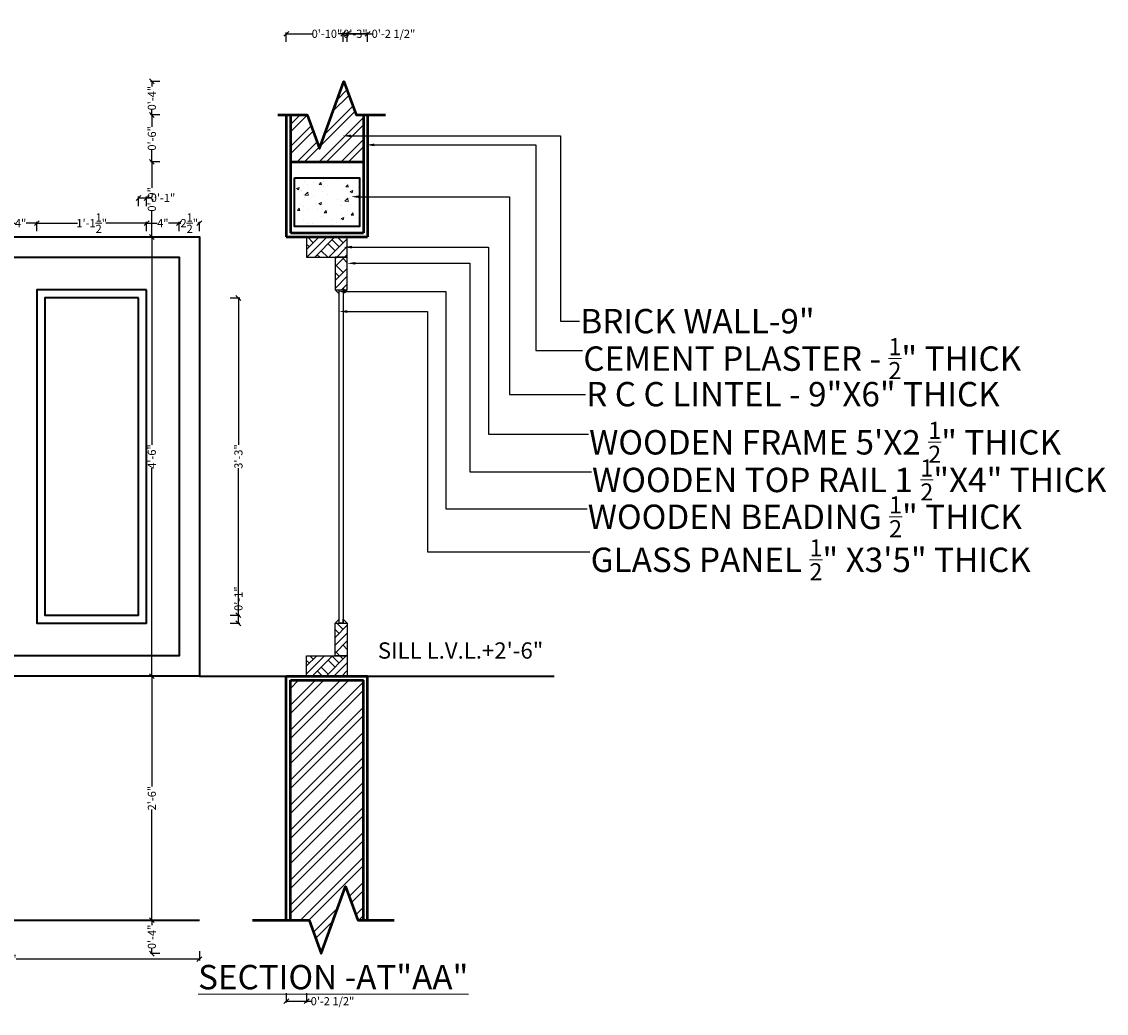
# Model space of a CAD drawing. Units: inches. Extents: x -54 to 163, y -154 to 48.
# Tile 3 of 3: x 30 to 163, y -74 to 48. Entities that reach past the tile are written whole.
import ezdxf
from ezdxf import colors
from ezdxf.entities.mleader import LeaderData, LeaderLine
from ezdxf.math import Vec2, Vec3

# ---------------------------------------------------------------- set-up
doc = ezdxf.new("R2010")
doc.units = ezdxf.units.IN
doc.header["$MEASUREMENT"] = 0
for name, color, linetype, lineweight in [('A-ANNO-DIMS', 2, 'Continuous', 18), ('A-ANNO-TEXT', 3, 'Continuous', 18), ('A-ELEV', 7, 'Continuous', 35), ('A-GLAZ', 4, 'Continuous', 25), ('A-GLAZ-PATT', 9, 'Continuous', 13), ('A-WALL', 7, 'Continuous', 50), ('A-WALL-PATT', 8, 'Continuous', 18), ('S-BEAM', 1, 'Continuous', 35)]:
    doc.layers.add(name, color=color, linetype=linetype, lineweight=lineweight)
doc.styles.get("Standard").update_dxf_attribs({"font": 'arial.ttf'})
doc.dimstyles.get("Standard").update_dxf_attribs({"dimtxt": 1, "dimasz": 0.6, "dimexe": 0.18, "dimexo": 0.0625, "dimgap": 0.09, "dimtad": 0, "dimdec": 1, "dimzin": 0, "dimdsep": 46, "dimlunit": 4, "dimtxsty": 'Standard', "dimblk": 'OBLIQUE', "dimcen": 0.09, "dimadec": 0, "dimazin": 0, "dimtfac": 1, "dimtdec": 1, "dimtofl": 0, "dimtmove": 0, "dimatfit": 3, "dimfxl": 1, "dimfxlon": 1, "dimtolj": 1, "dimtzin": 0, "dimarcsym": 0})

# ---------------------------------------------------------------- blocks, each defined once
blk = doc.blocks.new('_Oblique')
at = {"color": 0, "linetype": 'ByBlock', "lineweight": -2}
blk.add_line((-0.5, -0.5), (0.5, 0.5), dxfattribs=at)
blk = doc.blocks.new('*D6')
at = {"layer": 'A-ANNO-DIMS', "color": 0, "lineweight": -2, "transparency": 16777216}
for p, q in [((27.48, 22.51), (27.48, 23.69)), ((27.48, 23.51), (28.8, 23.51)), ((31.48, 23.51), (30.17, 23.51)), ((31.48, 22.51), (31.48, 23.69))]:
    blk.add_line(p, q, dxfattribs=at)
at = {"layer": 'Defpoints', "color": 0, "transparency": 16777216}
for p in [(31.48, 23.51), (27.48, 15.31), (31.48, 15.31)]:
    blk.add_point(p, dxfattribs=at)
at = {"layer": 'A-ANNO-DIMS', "color": 0, "lineweight": -2, "transparency": 16777216, "xscale": 0.6, "yscale": 0.6, "zscale": 0.6, "rotation": 180}
blk.add_blockref('_Oblique', (27.48, 23.51), dxfattribs=at)
at = {"layer": 'A-ANNO-DIMS', "color": 0, "lineweight": -2, "transparency": 16777216, "xscale": 0.6, "yscale": 0.6, "zscale": 0.6}
blk.add_blockref('_Oblique', (31.48, 23.51), dxfattribs=at)
at = {"layer": 'A-ANNO-DIMS', "color": 0, "transparency": 16777216, "insert": (29.48, 23.51), "char_height": 1, "attachment_point": 5}
blk.add_mtext('\\A1;4"', dxfattribs=at)
blk = doc.blocks.new('*D7')
at = {"layer": 'A-ANNO-DIMS', "color": 0, "lineweight": -2, "transparency": 16777216}
for p, q in [((31.48, 22.51), (31.48, 23.69)), ((31.48, 23.51), (36.49, 23.51)), ((44.98, 23.51), (39.97, 23.51)), ((44.98, 22.51), (44.98, 23.69))]:
    blk.add_line(p, q, dxfattribs=at)
at = {"layer": 'Defpoints', "color": 0, "transparency": 16777216}
for p in [(44.98, 23.51), (31.48, 15.31), (44.98, 15.31)]:
    blk.add_point(p, dxfattribs=at)
at = {"layer": 'A-ANNO-DIMS', "color": 0, "lineweight": -2, "transparency": 16777216, "xscale": 0.6, "yscale": 0.6, "zscale": 0.6, "rotation": 180}
blk.add_blockref('_Oblique', (31.48, 23.51), dxfattribs=at)
at = {"layer": 'A-ANNO-DIMS', "color": 0, "lineweight": -2, "transparency": 16777216, "xscale": 0.6, "yscale": 0.6, "zscale": 0.6}
blk.add_blockref('_Oblique', (44.98, 23.51), dxfattribs=at)
at = {"layer": 'A-ANNO-DIMS', "color": 0, "transparency": 16777216, "insert": (38.23, 23.51), "char_height": 1, "attachment_point": 5}
blk.add_mtext('\\A1;1\'-1{\\H1x;\\S1/2;}"', dxfattribs=at)
blk = doc.blocks.new('*D8')
at = {"layer": 'A-ANNO-DIMS', "color": 0, "lineweight": -2, "transparency": 16777216}
for p, q in [((44.98, 22.51), (44.98, 23.69)), ((44.98, 23.51), (46.3, 23.51)), ((48.98, 23.51), (47.67, 23.51)), ((48.98, 22.51), (48.98, 23.69))]:
    blk.add_line(p, q, dxfattribs=at)
at = {"layer": 'Defpoints', "color": 0, "transparency": 16777216}
for p in [(48.98, 23.51), (44.98, 15.31), (48.98, 15.31)]:
    blk.add_point(p, dxfattribs=at)
at = {"layer": 'A-ANNO-DIMS', "color": 0, "lineweight": -2, "transparency": 16777216, "xscale": 0.6, "yscale": 0.6, "zscale": 0.6, "rotation": 180}
blk.add_blockref('_Oblique', (44.98, 23.51), dxfattribs=at)
at = {"layer": 'A-ANNO-DIMS', "color": 0, "lineweight": -2, "transparency": 16777216, "xscale": 0.6, "yscale": 0.6, "zscale": 0.6}
blk.add_blockref('_Oblique', (48.98, 23.51), dxfattribs=at)
at = {"layer": 'A-ANNO-DIMS', "color": 0, "transparency": 16777216, "insert": (46.98, 23.51), "char_height": 1, "attachment_point": 5}
blk.add_mtext('\\A1;4"', dxfattribs=at)
blk = doc.blocks.new('*D9')
at = {"layer": 'A-ANNO-DIMS', "color": 0, "lineweight": -2, "transparency": 16777216}
for p, q in [((48.98, 22.51), (48.98, 23.69)), ((48.98, 23.51), (49.19, 23.51)), ((51.48, 23.51), (51.27, 23.51)), ((51.48, 22.51), (51.48, 23.69))]:
    blk.add_line(p, q, dxfattribs=at)
at = {"layer": 'Defpoints', "color": 0, "transparency": 16777216}
for p in [(51.48, 23.51), (48.98, 19.31), (51.48, 19.31)]:
    blk.add_point(p, dxfattribs=at)
at = {"layer": 'A-ANNO-DIMS', "color": 0, "lineweight": -2, "transparency": 16777216, "xscale": 0.6, "yscale": 0.6, "zscale": 0.6, "rotation": 180}
blk.add_blockref('_Oblique', (48.98, 23.51), dxfattribs=at)
at = {"layer": 'A-ANNO-DIMS', "color": 0, "lineweight": -2, "transparency": 16777216, "xscale": 0.6, "yscale": 0.6, "zscale": 0.6}
blk.add_blockref('_Oblique', (51.48, 23.51), dxfattribs=at)
at = {"layer": 'A-ANNO-DIMS', "color": 0, "transparency": 16777216, "insert": (50.23, 23.51), "char_height": 1, "attachment_point": 5}
blk.add_mtext('\\A1;2{\\H1x;\\S1/2;}"', dxfattribs=at)
blk = doc.blocks.new('*D18')
at = {"layer": 'A-ANNO-DIMS', "color": 0, "lineweight": -2, "transparency": 16777216}
for p, q in [((3.48, -65.99), (3.48, -67.17)), ((51.48, -65.99), (51.48, -67.17)), ((3.48, -66.99), (26.04, -66.99)), ((51.48, -66.99), (28.92, -66.99))]:
    blk.add_line(p, q, dxfattribs=at)
at = {"layer": 'Defpoints', "color": 0, "transparency": 16777216}
for p in [(3.48, -62.19), (51.48, -62.19), (51.48, -66.99)]:
    blk.add_point(p, dxfattribs=at)
at = {"layer": 'A-ANNO-DIMS', "color": 0, "lineweight": -2, "transparency": 16777216, "xscale": 0.6, "yscale": 0.6, "zscale": 0.6, "rotation": 180}
blk.add_blockref('_Oblique', (3.48, -66.99), dxfattribs=at)
at = {"layer": 'A-ANNO-DIMS', "color": 0, "lineweight": -2, "transparency": 16777216, "xscale": 0.6, "yscale": 0.6, "zscale": 0.6}
blk.add_blockref('_Oblique', (51.48, -66.99), dxfattribs=at)
at = {"layer": 'A-ANNO-DIMS', "color": 0, "transparency": 16777216, "insert": (27.48, -66.99), "char_height": 1, "attachment_point": 5}
blk.add_mtext('\\A1;4\'-0"', dxfattribs=at)
blk = doc.blocks.new('*D20')
at = {"layer": 'A-ANNO-DIMS', "color": 0, "lineweight": -2, "transparency": 16777216}
for p, q in [((55.28, 14.31), (56.46, 14.31)), ((56.28, 14.31), (56.28, -3.77)), ((56.28, -24.69), (56.28, -6.6)), ((55.28, -24.69), (56.46, -24.69))]:
    blk.add_line(p, q, dxfattribs=at)
at = {"layer": 'Defpoints', "color": 0, "transparency": 16777216}
for p in [(10.98, 14.31), (10.98, -24.69), (56.28, -24.69)]:
    blk.add_point(p, dxfattribs=at)
at = {"layer": 'A-ANNO-DIMS', "color": 0, "lineweight": -2, "transparency": 16777216, "xscale": 0.6, "yscale": 0.6, "zscale": 0.6}
for p, rotation in [((56.28, 14.31), 90), ((56.28, -24.69), 270)]:
    blk.add_blockref('_Oblique', p, dxfattribs=dict(at, rotation=rotation))
at = {"layer": 'A-ANNO-DIMS', "color": 0, "transparency": 16777216, "insert": (56.28, -5.19), "char_height": 1, "attachment_point": 5, "rotation": 90}
blk.add_mtext('\\A1;3\'-3"', dxfattribs=at)
blk = doc.blocks.new('*D21')
at = {"layer": 'A-ANNO-DIMS', "color": 0, "lineweight": -2, "transparency": 16777216}
for p, q in [((43.98, 25.61), (43.98, 26.79)), ((44.98, 25.61), (44.98, 26.79)), ((43.98, 26.61), (44.98, 26.61)), ((44.98, 26.61), (45.58, 26.61))]:
    blk.add_line(p, q, dxfattribs=at)
at = {"layer": 'Defpoints', "color": 0, "transparency": 16777216}
for p in [(44.98, 26.61), (44.98, 15.31), (43.98, 14.31)]:
    blk.add_point(p, dxfattribs=at)
at = {"layer": 'A-ANNO-DIMS', "color": 0, "lineweight": -2, "transparency": 16777216, "xscale": 0.6, "yscale": 0.6, "zscale": 0.6, "rotation": 180}
blk.add_blockref('_Oblique', (43.98, 26.61), dxfattribs=at)
at = {"layer": 'A-ANNO-DIMS', "color": 0, "lineweight": -2, "transparency": 16777216, "xscale": 0.6, "yscale": 0.6, "zscale": 0.6}
blk.add_blockref('_Oblique', (44.98, 26.61), dxfattribs=at)
at = {"layer": 'A-ANNO-DIMS', "color": 0, "transparency": 16777216, "insert": (47, 26.61), "char_height": 1, "attachment_point": 5}
blk.add_mtext('\\A1;0\'-1"', dxfattribs=at)
blk = doc.blocks.new('*D22')
at = {"layer": 'A-ANNO-DIMS', "color": 0, "lineweight": -2, "transparency": 16777216}
for p, q in [((55.28, -24.69), (56.46, -24.69)), ((56.28, -24.69), (56.28, -24.09)), ((56.28, -25.69), (56.28, -24.69)), ((55.28, -25.69), (56.46, -25.69))]:
    blk.add_line(p, q, dxfattribs=at)
at = {"layer": 'Defpoints', "color": 0, "transparency": 16777216}
for p in [(43.98, -24.69), (56.28, -24.69), (44.98, -25.69)]:
    blk.add_point(p, dxfattribs=at)
at = {"layer": 'A-ANNO-DIMS', "color": 0, "lineweight": -2, "transparency": 16777216, "xscale": 0.6, "yscale": 0.6, "zscale": 0.6}
for p, rotation in [((56.28, -24.69), 90), ((56.28, -25.69), 270)]:
    blk.add_blockref('_Oblique', p, dxfattribs=dict(at, rotation=rotation))
at = {"layer": 'A-ANNO-DIMS', "color": 0, "transparency": 16777216, "insert": (56.28, -22.67), "char_height": 1, "attachment_point": 5, "rotation": 90}
blk.add_mtext('\\A1;0\'-1"', dxfattribs=at)
blk = doc.blocks.new('*D23')
at = {"layer": 'A-ANNO-DIMS', "color": 0, "lineweight": -2, "transparency": 16777216}
for p, q in [((62.17, 45.79), (62.17, 46.97)), ((62.17, 46.79), (65.36, 46.79)), ((72.17, 46.79), (68.97, 46.79)), ((72.17, 45.79), (72.17, 46.97))]:
    blk.add_line(p, q, dxfattribs=at)
at = {"layer": 'Defpoints', "color": 0, "transparency": 16777216}
for p in [(72.17, 46.79), (62.17, 36.81), (72.17, 36.81)]:
    blk.add_point(p, dxfattribs=at)
at = {"layer": 'A-ANNO-DIMS', "color": 0, "lineweight": -2, "transparency": 16777216, "xscale": 0.6, "yscale": 0.6, "zscale": 0.6, "rotation": 180}
blk.add_blockref('_Oblique', (62.17, 46.79), dxfattribs=at)
at = {"layer": 'A-ANNO-DIMS', "color": 0, "lineweight": -2, "transparency": 16777216, "xscale": 0.6, "yscale": 0.6, "zscale": 0.6}
blk.add_blockref('_Oblique', (72.17, 46.79), dxfattribs=at)
at = {"layer": 'A-ANNO-DIMS', "color": 0, "transparency": 16777216, "insert": (67.17, 46.79), "char_height": 1, "attachment_point": 5}
blk.add_mtext('\\A1;0\'-10"', dxfattribs=at)
blk = doc.blocks.new('*D24')
at = {"layer": 'A-ANNO-DIMS', "color": 0, "lineweight": -2, "transparency": 16777216}
for p, q in [((46.63, 40.94), (45.45, 40.94)), ((45.63, 40.94), (45.63, 40.29)), ((45.63, 36.81), (45.63, 37.46)), ((46.63, 36.81), (45.45, 36.81))]:
    blk.add_line(p, q, dxfattribs=at)
at = {"layer": 'Defpoints', "color": 0, "transparency": 16777216}
for p in [(69.25, 40.94), (45.63, 36.81), (62.17, 36.81)]:
    blk.add_point(p, dxfattribs=at)
at = {"layer": 'A-ANNO-DIMS', "color": 0, "lineweight": -2, "transparency": 16777216, "xscale": 0.6, "yscale": 0.6, "zscale": 0.6}
for p, rotation in [((45.63, 40.94), 90), ((45.63, 36.81), 270)]:
    blk.add_blockref('_Oblique', p, dxfattribs=dict(at, rotation=rotation))
at = {"layer": 'A-ANNO-DIMS', "color": 0, "transparency": 16777216, "insert": (45.63, 38.88), "char_height": 1, "attachment_point": 5, "rotation": 90}
blk.add_mtext('\\A1;0\'-4"', dxfattribs=at)
blk = doc.blocks.new('*D25')
at = {"layer": 'A-ANNO-DIMS', "color": 0, "lineweight": -2, "transparency": 16777216}
for p, q in [((46.63, 36.81), (45.45, 36.81)), ((45.63, 36.81), (45.63, 35.35)), ((45.63, 31.05), (45.63, 32.51)), ((46.63, 31.05), (45.45, 31.05))]:
    blk.add_line(p, q, dxfattribs=at)
at = {"layer": 'Defpoints', "color": 0, "transparency": 16777216}
for p in [(62.17, 36.81), (45.63, 31.05), (62.67, 31.05)]:
    blk.add_point(p, dxfattribs=at)
at = {"layer": 'A-ANNO-DIMS', "color": 0, "lineweight": -2, "transparency": 16777216, "xscale": 0.6, "yscale": 0.6, "zscale": 0.6}
for p, rotation in [((45.63, 36.81), 90), ((45.63, 31.05), 270)]:
    blk.add_blockref('_Oblique', p, dxfattribs=dict(at, rotation=rotation))
at = {"layer": 'A-ANNO-DIMS', "color": 0, "transparency": 16777216, "insert": (45.63, 33.93), "char_height": 1, "attachment_point": 5, "rotation": 90}
blk.add_mtext('\\A1;0\'-6"', dxfattribs=at)
blk = doc.blocks.new('*D26')
at = {"layer": 'A-ANNO-DIMS', "color": 0, "lineweight": -2, "transparency": 16777216}
for p, q in [((46.63, 31.05), (45.45, 31.05)), ((45.63, 31.05), (45.63, 27.85)), ((45.63, 21.81), (45.63, 25.01)), ((46.63, 21.81), (45.45, 21.81))]:
    blk.add_line(p, q, dxfattribs=at)
at = {"layer": 'Defpoints', "color": 0, "transparency": 16777216}
for p in [(62.67, 31.05), (45.63, 21.81), (62.17, 21.81)]:
    blk.add_point(p, dxfattribs=at)
at = {"layer": 'A-ANNO-DIMS', "color": 0, "lineweight": -2, "transparency": 16777216, "xscale": 0.6, "yscale": 0.6, "zscale": 0.6}
for p, rotation in [((45.63, 31.05), 90), ((45.63, 21.81), 270)]:
    blk.add_blockref('_Oblique', p, dxfattribs=dict(at, rotation=rotation))
at = {"layer": 'A-ANNO-DIMS', "color": 0, "transparency": 16777216, "insert": (45.63, 26.43), "char_height": 1, "attachment_point": 5, "rotation": 90}
blk.add_mtext('\\A1;0\'-9"', dxfattribs=at)
blk = doc.blocks.new('*D27')
at = {"layer": 'A-ANNO-DIMS', "color": 0, "lineweight": -2, "transparency": 16777216}
for p, q in [((46.63, 21.81), (45.45, 21.81)), ((45.63, 21.81), (45.63, -3.75)), ((45.63, -32.19), (45.63, -6.62)), ((46.63, -32.19), (45.45, -32.19))]:
    blk.add_line(p, q, dxfattribs=at)
at = {"layer": 'Defpoints', "color": 0, "transparency": 16777216}
for p in [(62.17, 21.81), (45.63, -32.19), (62.17, -32.19)]:
    blk.add_point(p, dxfattribs=at)
at = {"layer": 'A-ANNO-DIMS', "color": 0, "lineweight": -2, "transparency": 16777216, "xscale": 0.6, "yscale": 0.6, "zscale": 0.6}
for p, rotation in [((45.63, 21.81), 90), ((45.63, -32.19), 270)]:
    blk.add_blockref('_Oblique', p, dxfattribs=dict(at, rotation=rotation))
at = {"layer": 'A-ANNO-DIMS', "color": 0, "transparency": 16777216, "insert": (45.63, -5.19), "char_height": 1, "attachment_point": 5, "rotation": 90}
blk.add_mtext('\\A1;4\'-6"', dxfattribs=at)
blk = doc.blocks.new('*D28')
at = {"layer": 'A-ANNO-DIMS', "color": 0, "lineweight": -2, "transparency": 16777216}
for p, q in [((46.63, -32.19), (45.45, -32.19)), ((45.63, -32.19), (45.63, -45.76)), ((45.63, -62.19), (45.63, -48.61)), ((46.63, -62.19), (45.45, -62.19))]:
    blk.add_line(p, q, dxfattribs=at)
at = {"layer": 'Defpoints', "color": 0, "transparency": 16777216}
for p in [(62.17, -32.19), (45.63, -62.19), (62.17, -62.19)]:
    blk.add_point(p, dxfattribs=at)
at = {"layer": 'A-ANNO-DIMS', "color": 0, "lineweight": -2, "transparency": 16777216, "xscale": 0.6, "yscale": 0.6, "zscale": 0.6}
for p, rotation in [((45.63, -32.19), 90), ((45.63, -62.19), 270)]:
    blk.add_blockref('_Oblique', p, dxfattribs=dict(at, rotation=rotation))
at = {"layer": 'A-ANNO-DIMS', "color": 0, "transparency": 16777216, "insert": (45.63, -47.19), "char_height": 1, "attachment_point": 5, "rotation": 90}
blk.add_mtext('\\A1;2\'-6"', dxfattribs=at)
blk = doc.blocks.new('*D29')
at = {"layer": 'A-ANNO-DIMS', "color": 0, "lineweight": -2, "transparency": 16777216}
for p, q in [((46.63, -62.19), (45.45, -62.19)), ((45.63, -62.19), (45.63, -62.83)), ((46.63, -66.31), (45.45, -66.31)), ((45.63, -66.31), (45.63, -65.67))]:
    blk.add_line(p, q, dxfattribs=at)
at = {"layer": 'Defpoints', "color": 0, "transparency": 16777216}
for p in [(62.17, -62.19), (45.63, -66.31), (66.46, -66.31)]:
    blk.add_point(p, dxfattribs=at)
at = {"layer": 'A-ANNO-DIMS', "color": 0, "lineweight": -2, "transparency": 16777216, "xscale": 0.6, "yscale": 0.6, "zscale": 0.6}
for p, rotation in [((45.63, -62.19), 90), ((45.63, -66.31), 270)]:
    blk.add_blockref('_Oblique', p, dxfattribs=dict(at, rotation=rotation))
at = {"layer": 'A-ANNO-DIMS', "color": 0, "transparency": 16777216, "insert": (45.63, -64.25), "char_height": 1, "attachment_point": 5, "rotation": 90}
blk.add_mtext('\\A1;0\'-4"', dxfattribs=at)
blk = doc.blocks.new('*D30')
at = {"layer": 'A-ANNO-DIMS', "color": 0, "lineweight": -2, "transparency": 16777216}
for p, q in [((69.67, 45.79), (69.67, 46.97)), ((69.67, 46.79), (72.17, 46.79)), ((72.17, 45.79), (72.17, 46.97)), ((72.17, 46.79), (72.77, 46.79))]:
    blk.add_line(p, q, dxfattribs=at)
at = {"layer": 'Defpoints', "color": 0, "transparency": 16777216}
for p in [(72.17, 46.79), (69.67, -32.19), (72.17, -32.19)]:
    blk.add_point(p, dxfattribs=at)
at = {"layer": 'A-ANNO-DIMS', "color": 0, "lineweight": -2, "transparency": 16777216, "xscale": 0.6, "yscale": 0.6, "zscale": 0.6, "rotation": 180}
blk.add_blockref('_Oblique', (69.67, 46.79), dxfattribs=at)
at = {"layer": 'A-ANNO-DIMS', "color": 0, "lineweight": -2, "transparency": 16777216, "xscale": 0.6, "yscale": 0.6, "zscale": 0.6}
blk.add_blockref('_Oblique', (72.17, 46.79), dxfattribs=at)
at = {"layer": 'A-ANNO-DIMS', "color": 0, "transparency": 16777216, "insert": (75.35, 46.79), "char_height": 1, "attachment_point": 5}
blk.add_mtext('\\A1;0\'-2 1/2"', dxfattribs=at)
blk = doc.blocks.new('*D31')
at = {"layer": 'A-ANNO-DIMS', "color": 0, "lineweight": -2, "transparency": 16777216}
for p, q in [((69.165189, 46.786945), (68.565189, 46.786945)), ((69.165189, 45.786945), (69.165189, 46.966945)), ((72.165189, 45.786945), (72.165189, 46.966945)), ((72.165189, 46.786945), (72.765189, 46.786945))]:
    blk.add_line(p, q, dxfattribs=at)
at = {"layer": 'Defpoints', "color": 0, "transparency": 16777216}
for p in [(72.165189, 46.786945), (69.165189, -25.685371), (72.165189, -32.185371)]:
    blk.add_point(p, dxfattribs=at)
at = {"layer": 'A-ANNO-DIMS', "color": 0, "lineweight": -2, "transparency": 16777216, "xscale": 0.6, "yscale": 0.6, "zscale": 0.6}
blk.add_blockref('_Oblique', (69.165189, 46.786945), dxfattribs=at)
at = {"layer": 'A-ANNO-DIMS', "color": 0, "lineweight": -2, "transparency": 16777216, "xscale": 0.6, "yscale": 0.6, "zscale": 0.6, "rotation": 180}
blk.add_blockref('_Oblique', (72.165189, 46.786945), dxfattribs=at)
at = {"layer": 'A-ANNO-DIMS', "color": 0, "transparency": 16777216, "insert": (70.665189, 46.786945), "char_height": 1, "attachment_point": 5}
blk.add_mtext('\\A1;0\'-3"', dxfattribs=at)
blk = doc.blocks.new('*D32')
at = {"layer": 'A-ANNO-DIMS', "color": 0, "lineweight": -2, "transparency": 16777216}
for p, q in [((62.17, -71.16), (62.17, -72.34)), ((64.67, -71.16), (64.67, -72.34)), ((62.17, -72.16), (64.67, -72.16)), ((64.67, -72.16), (65.27, -72.16))]:
    blk.add_line(p, q, dxfattribs=at)
at = {"layer": 'Defpoints', "color": 0, "transparency": 16777216}
for p in [(62.17, 21.81), (64.67, 21.81), (64.67, -72.16)]:
    blk.add_point(p, dxfattribs=at)
at = {"layer": 'A-ANNO-DIMS', "color": 0, "lineweight": -2, "transparency": 16777216, "xscale": 0.6, "yscale": 0.6, "zscale": 0.6, "rotation": 180}
blk.add_blockref('_Oblique', (62.17, -72.16), dxfattribs=at)
at = {"layer": 'A-ANNO-DIMS', "color": 0, "lineweight": -2, "transparency": 16777216, "xscale": 0.6, "yscale": 0.6, "zscale": 0.6}
blk.add_blockref('_Oblique', (64.67, -72.16), dxfattribs=at)
at = {"layer": 'A-ANNO-DIMS', "color": 0, "transparency": 16777216, "insert": (67.85, -72.16), "char_height": 1, "attachment_point": 5}
blk.add_mtext('\\A1;0\'-2 1/2"', dxfattribs=at)

msp = doc.modelspace()

# ---------------------------------------------------------------- hatches: boundary and pattern name
at = {"layer": 'A-GLAZ-PATT'}
h = msp.add_hatch(dxfattribs=at)
h.set_pattern_fill('º»ÊµÍÁÈÀ', color=256, scale=0.46)
h.set_pattern_definition([(45, (0.5428, 0), (-1.82801, 1.82801), []), (45, (1.5088, 0), (-1.82801, 1.82801), []), (45, (2.4748, 0), (-1.82801, 1.82801), []), (135, (0.5428, 0), (-1.82801, -1.82801), [1.219, -1.3662]), (135, (1.0258, 0.483), (-1.82801, -1.82801), [1.219, -1.3662]), (135, (1.5088, 0.966), (-1.82801, -1.82801), [1.219, -1.3662])])
h.paths.add_polyline_path([(69.67, 21.81), (64.67, 21.81), (64.67, 19.31), (69.67, 19.31)])
h.paths.add_polyline_path([(68.17, 15.31), (69.67, 15.31), (69.67, 19.31), (68.17, 19.31)])
h.paths.add_polyline_path([(68.17, -29.69), (64.67, -29.69), (64.67, -32.19), (69.67, -32.19), (69.67, -29.69)])
h.paths.add_polyline_path([(69.67, -25.69), (68.17, -25.69), (68.17, -29.69), (69.67, -29.69)])
at = {"layer": 'A-WALL-PATT'}
h = msp.add_hatch(dxfattribs=at)
h.set_pattern_fill('ANSI32', color=256, scale=5.1)
h.paths.add_polyline_path([(71.67, 36.81), (70.75, 36.81), (69.25, 40.94), (66.25, 32.69), (64.75, 36.81), (62.67, 36.81), (62.67, 31.05), (71.67, 31.05)])
h = msp.add_hatch(dxfattribs=at)
h.set_pattern_fill('AR-CONC', color=256, scale=0.46)
h.paths.add_polyline_path([(71.18, 29.08), (63.18, 29.08), (63.18, 23.08), (71.18, 23.08)])
h = msp.add_hatch(dxfattribs=at)
h.set_pattern_fill('ANSI32', color=256, scale=5.8)
h.paths.add_polyline_path([(71.67, -32.69), (62.67, -32.69), (62.67, -62.19), (64.96, -62.19), (66.46, -66.31), (69.46, -58.06), (70.96, -62.19), (71.67, -62.19)])

# ---------------------------------------------------------------- linework, layer by layer
at = {"layer": 'A-ELEV'}
for p, q in [((51.48, -32.19), (95.13, -32.19)), ((-20.18, -62.19), (51.48, -62.19))]:
    msp.add_line(p, q, dxfattribs=at)
msp.add_lwpolyline([(3.48, 21.81), (51.48, 21.81), (51.48, 19.31), (51.48, -29.69), (51.48, -32.19), (3.48, -32.19), (3.48, 21.81)], dxfattribs=at)
for points in [[(5.98, 19.31), (48.98, 19.31), (48.98, -29.69), (5.98, -29.69)], [(44.98, 15.31), (31.48, 15.31), (31.48, -25.69), (44.98, -25.69)], [(43.98, 14.31), (32.48, 14.31), (32.48, -24.69), (43.98, -24.69)]]:
    msp.add_lwpolyline(points, close=True, dxfattribs=at)
at = {"layer": 'A-GLAZ'}
for p, q in [((68.67, 14.81), (68.17, 15.31)), ((69.17, 14.81), (69.67, 15.31)), ((68.67, -25.19), (68.17, -25.69)), ((69.17, -25.69), (69.17, -25.19)), ((69.17, -25.19), (69.67, -25.69))]:
    msp.add_line(p, q, dxfattribs=at)
for points in [[(64.67, 19.31), (69.67, 19.31), (69.67, 21.81), (64.67, 21.81)], [(68.17, 15.31), (69.67, 15.31), (69.67, 19.31), (68.17, 19.31)], [(68.67, 15.31), (69.17, 15.31), (69.17, -25.69), (68.67, -25.69)], [(68.17, -25.69), (69.67, -25.69), (69.67, -29.69), (68.17, -29.69)], [(64.67, -29.69), (69.67, -29.69), (69.67, -32.19), (64.67, -32.19)]]:
    msp.add_lwpolyline(points, close=True, dxfattribs=at)
at = {"layer": 'A-WALL'}
for p, q in [((62.17, 36.81), (62.17, 21.81)), ((62.67, 36.81), (62.67, 22.31)), ((71.67, 36.81), (71.67, 22.31)), ((72.17, 36.81), (72.17, 21.81)), ((62.67, 31.05), (71.67, 31.05)), ((62.17, 21.81), (72.17, 21.81)), ((62.67, 22.31), (71.67, 22.31)), ((62.17, -62.19), (62.17, -32.19)), ((62.17, -32.19), (72.17, -32.19)), ((62.67, -62.19), (62.67, -32.69)), ((62.67, -32.69), (71.67, -32.69)), ((71.67, -62.19), (71.67, -32.69)), ((72.17, -62.19), (72.17, -32.19))]:
    msp.add_line(p, q, dxfattribs=at)
for points in [[(61.14, 36.81), (64.75, 36.81), (66.25, 32.69), (69.25, 40.94), (70.75, 36.81), (74.37, 36.81)], [(58.01, -62.19), (64.96, -62.19), (66.46, -66.31), (69.46, -58.06), (70.96, -62.19), (75.42, -62.19)]]:
    msp.add_lwpolyline(points, dxfattribs=at)
at = {"layer": 'S-BEAM'}
msp.add_lwpolyline([(63.18, 29.08), (71.18, 29.08), (71.18, 23.08), (63.18, 23.08)], close=True, dxfattribs=at)

# ---------------------------------------------------------------- texts
at = {"layer": 'A-ANNO-TEXT', "attachment_point": 1}
for s, width, insert, char_height in [('SILL L.V.L.+2\'-6"', 31.9073, (73.43, -28.04), 2), ('{\\LSECTION -AT"AA"}', 38.8682, (51.32, -67.7), 3)]:
    msp.add_mtext_dynamic_manual_height_columns(s, width=width, gutter_width=1, heights=[0], dxfattribs=dict(at, insert=insert, char_height=char_height))

# ---------------------------------------------------------------- dimensions: what is measured, and where the dimension line sits
at = {"layer": 'A-ANNO-DIMS'}
for base, p1, p2, override, picture, middle in [((72.17, 46.79), (69.67, -32.19), (72.17, -32.19), {"dimdec": 1, "dimlfac": 1, "dimrnd": 0, "dimzin": 1, "dimdsep": 46, "dimlunit": 4, "dimfrac": 2}, '*D30', (75.35, 46.79)), ((72.17, 46.79), (62.17, 36.81), (72.17, 36.81), {"dimdec": 1, "dimlfac": 1, "dimrnd": 0, "dimzin": 1, "dimdsep": 46, "dimlunit": 4, "dimfrac": 2}, '*D23', (67.17, 46.79)), ((72.17, 46.79), (69.17, -25.69), (72.17, -32.19), {"dimdec": 1, "dimlfac": 1, "dimrnd": 0, "dimzin": 1, "dimdsep": 46, "dimlunit": 4, "dimfrac": 2}, '*D31', (70.67, 46.79)), ((44.98, 26.61), (43.98, 14.31), (44.98, 15.31), {"dimdec": 1, "dimlfac": 1, "dimrnd": 0, "dimzin": 1, "dimdsep": 46, "dimlunit": 4, "dimfrac": 2}, '*D21', (47, 26.61)), ((31.48, 23.51), (27.48, 15.31), (31.48, 15.31), {"dimclrd": 0, "dimclre": 0, "dimclrt": 0}, '*D6', (29.48, 23.51)), ((44.98, 23.51), (31.48, 15.31), (44.98, 15.31), {"dimclrd": 0, "dimclre": 0, "dimclrt": 0}, '*D7', (38.23, 23.51)), ((48.98, 23.51), (44.98, 15.31), (48.98, 15.31), {"dimclrd": 0, "dimclre": 0, "dimclrt": 0}, '*D8', (46.98, 23.51)), ((51.48, 23.51), (48.98, 19.31), (51.48, 19.31), {"dimclrd": 0, "dimclre": 0, "dimclrt": 0}, '*D9', (50.23, 23.51)), ((64.67, -72.16), (62.17, 21.81), (64.67, 21.81), {"dimdec": 1, "dimlfac": 1, "dimrnd": 0, "dimzin": 1, "dimdsep": 46, "dimlunit": 4, "dimfrac": 2}, '*D32', (67.85, -72.16)), ((51.48, -66.99), (3.48, -62.19), (51.48, -62.19), {"dimdec": 1, "dimlfac": 1, "dimrnd": 0, "dimzin": 1, "dimdsep": 46, "dimlunit": 4, "dimfrac": 2}, '*D18', (27.48, -66.99))]:
    dim = msp.add_linear_dim(base=base, p1=p1, p2=p2, dimstyle='Standard', override=override, dxfattribs=at)
    dim.commit()
    dim.dimension.update_dxf_attribs({"geometry": picture, "text_midpoint": middle})
for base, p1, p2, picture, middle in [((45.63, 36.81), (69.25, 40.94), (62.17, 36.81), '*D24', (45.63, 38.88)), ((45.63, 31.05), (62.17, 36.81), (62.67, 31.05), '*D25', (45.63, 33.93)), ((45.63, 21.81), (62.67, 31.05), (62.17, 21.81), '*D26', (45.63, 26.43)), ((45.63, -32.19), (62.17, 21.81), (62.17, -32.19), '*D27', (45.63, -5.19)), ((56.28, -24.69), (10.98, 14.31), (10.98, -24.69), '*D20', (56.28, -5.19)), ((56.28, -24.69), (44.98, -25.69), (43.98, -24.69), '*D22', (56.28, -22.67)), ((45.63, -62.19), (62.17, -32.19), (62.17, -62.19), '*D28', (45.63, -47.19)), ((45.63, -66.31), (62.17, -62.19), (66.46, -66.31), '*D29', (45.63, -64.25))]:
    dim = msp.add_linear_dim(base=base, p1=p1, p2=p2, angle=90, dimstyle='Standard', override={"dimdec": 1, "dimlfac": 1, "dimrnd": 0, "dimzin": 1, "dimdsep": 46, "dimlunit": 4, "dimfrac": 2}, dxfattribs=at)
    dim.commit()
    dim.dimension.update_dxf_attribs({"geometry": picture, "text_midpoint": middle})

# ---------------------------------------------------------------- leaders
at = {"layer": 'A-ANNO-TEXT'}
ml = msp.add_multileader_mtext('Standard', dxfattribs=at)
ml.set_content('BRICK WALL-9"', color=256)
ml.set_leader_properties()
ml.build(insert=Vec2(0, 0))
ml.multileader.update_dxf_attribs({"dogleg_length": 0.36, "arrow_head_size": 1})
ctx = ml.context
ctx.base_point, ctx.char_height, ctx.arrow_head_size, ctx.landing_gap_size, ctx.plane_origin = Vec3(98.25, 11.44), 3, 1, 0.09, Vec3(69.13, 34.24)
notes = []
notes.append((ctx, [(0, (1, 1, 0), (97.89, 11.44), (1, 0), 0.36, [(0, [(69.13, 34.24), (95.88, 34.24), (95.88, 11.44)], 0, [])])]))
ctx.mtext.insert, ctx.mtext.flow_direction = Vec3(98.34, 12.96), 5
ml = msp.add_multileader_mtext('Standard', dxfattribs=at)
ml.set_content('\\A1;CEMENT PLASTER - {\\H0.7x;\\S1/2;}" THICK', color=256)
ml.set_leader_properties()
ml.build(insert=Vec2(0, 0))
ml.multileader.update_dxf_attribs({"dogleg_length": 0.36, "arrow_head_size": 1})
ctx = ml.context
ctx.base_point, ctx.char_height, ctx.arrow_head_size, ctx.landing_gap_size, ctx.plane_origin = Vec3(98.61, 7.85), 3, 1, 0.09, Vec3(72, 33.13)
notes.append((ctx, [(0, (1, 1, 0), (98.25, 7.85), (1, 0), 0.36, [(0, [(72, 33.13), (92.86, 33.13), (92.86, 7.85)], 0, [])])]))
ctx.mtext.insert, ctx.mtext.flow_direction = Vec3(98.7, 9.37), 5
ml = msp.add_multileader_mtext('Standard', dxfattribs=at)
ml.set_content('R C C LINTEL - 9"X6" THICK', color=256)
ml.set_leader_properties()
ml.build(insert=Vec2(0, 0))
ml.multileader.update_dxf_attribs({"dogleg_length": 0.36, "arrow_head_size": 1})
ctx = ml.context
ctx.base_point, ctx.char_height, ctx.arrow_head_size, ctx.landing_gap_size, ctx.plane_origin = Vec3(98.97, 2.45), 3, 1, 0.09, Vec3(70.14, 26.76)
notes.append((ctx, [(0, (1, 1, 0), (98.61, 2.45), (1, 0), 0.36, [(0, [(70.14, 26.76), (89.64, 26.76), (89.64, 2.45)], 0, [])])]))
ctx.mtext.insert, ctx.mtext.flow_direction = Vec3(99.06, 3.98), 5
ml = msp.add_multileader_mtext('Standard', dxfattribs=at)
ml.set_content('\\A1;WOODEN FRAME 5\'X2 {\\H0.7x;\\S1/2;}" THICK', color=256)
ml.set_leader_properties()
ml.build(insert=Vec2(0, 0))
ml.multileader.update_dxf_attribs({"dogleg_length": 0.36, "arrow_head_size": 1})
ctx = ml.context
ctx.base_point, ctx.char_height, ctx.arrow_head_size, ctx.landing_gap_size, ctx.plane_origin = Vec3(99.33, -2.45), 3, 1, 0.09, Vec3(69.23, 20.56)
notes.append((ctx, [(0, (1, 1, 0), (98.97, -2.45), (1, 0), 0.36, [(0, [(69.23, 20.56), (87.03, 20.56), (87.03, -2.45)], 0, [])])]))
ctx.mtext.insert, ctx.mtext.flow_direction = Vec3(99.42, -0.92), 5
ml = msp.add_multileader_mtext('Standard', dxfattribs=at)
ml.set_content('\\A1;WOODEN TOP RAIL 1 {\\H0.7x;\\S1/2;}"X4" THICK', color=256)
ml.set_leader_properties()
ml.build(insert=Vec2(0, 0))
ml.multileader.update_dxf_attribs({"dogleg_length": 0.36, "arrow_head_size": 1})
ctx = ml.context
ctx.base_point, ctx.char_height, ctx.arrow_head_size, ctx.landing_gap_size, ctx.plane_origin = Vec3(99.69, -7.07), 3, 1, 0.09, Vec3(69.67, 18.57)
notes.append((ctx, [(0, (1, 1, 0), (99.33, -7.07), (1, 0), 0.36, [(0, [(69.67, 18.57), (84.75, 18.57), (84.75, -7.07)], 0, [])])]))
ctx.mtext.insert, ctx.mtext.flow_direction = Vec3(99.78, -5.55), 5
ml = msp.add_multileader_mtext('Standard', dxfattribs=at)
ml.set_content('\\A1;WOODEN BEADING {\\H0.7x;\\S1/2;}" THICK', color=256)
ml.set_leader_properties()
ml.build(insert=Vec2(0, 0))
ml.multileader.update_dxf_attribs({"dogleg_length": 0.36, "arrow_head_size": 1})
ctx = ml.context
ctx.base_point, ctx.char_height, ctx.arrow_head_size, ctx.landing_gap_size, ctx.plane_origin = Vec3(99.16, -11.61), 3, 1, 0.09, Vec3(68.52, 15.09)
notes.append((ctx, [(0, (1, 1, 0), (98.8, -11.61), (1, 0), 0.36, [(0, [(68.52, 15.09), (81.8, 15.09), (81.8, -11.64)], 0, [])])]))
ctx.mtext.insert, ctx.mtext.flow_direction = Vec3(99.25, -10.08), 5
ml = msp.add_multileader_mtext('Standard', dxfattribs=at)
ml.set_content('\\A1;GLASS PANEL {\\H0.7x;\\S1/2;}" X3\'5" THICK', color=256)
ml.set_leader_properties()
ml.build(insert=Vec2(0, 0))
ml.multileader.update_dxf_attribs({"dogleg_length": 0.36, "arrow_head_size": 1})
ctx = ml.context
ctx.base_point, ctx.char_height, ctx.arrow_head_size, ctx.landing_gap_size, ctx.plane_origin = Vec3(99.52, -16.9), 3, 1, 0.09, Vec3(68.67, 12.64)
notes.append((ctx, [(0, (1, 1, 0), (99.16, -16.9), (1, 0), 0.36, [(0, [(68.67, 12.64), (79.55, 12.64), (79.55, -16.9)], 0, [])])]))
ctx.mtext.insert, ctx.mtext.flow_direction = Vec3(99.61, -15.37), 5
for ctx, leaders in notes:
    for number, flags, end, landing, length, lines in leaders:
        leader = LeaderData()
        leader.index, (leader.has_last_leader_line, leader.has_dogleg_vector, leader.attachment_direction) = number, flags
        leader.last_leader_point, leader.dogleg_vector, leader.dogleg_length = Vec3(end), Vec3(landing), length
        for number, points, colour, breaks in lines:
            line = LeaderLine()
            line.index, line.vertices, line.color, line.breaks = number, Vec3.list(points), colors.encode_raw_color(colour), breaks
            leader.lines.append(line)
        ctx.leaders.append(leader)

doc.saveas('drawing.dxf')
